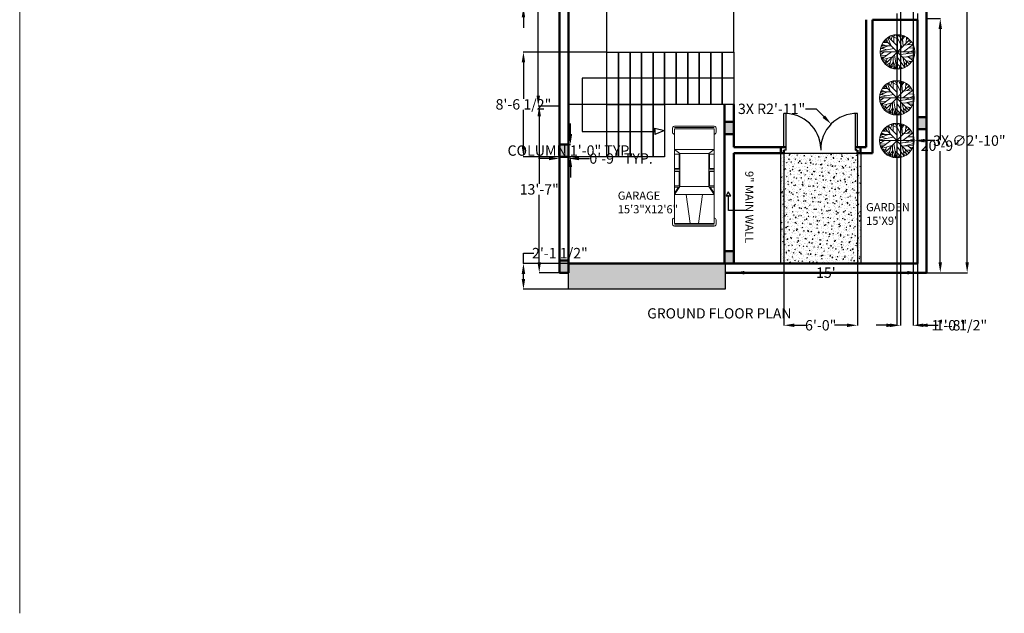
# Model space of a CAD drawing. Units: inches. Extents: x 22 to 1000, y 8 to 1043.
# Tile 1 of 3: x 22 to 987, y 8 to 590. Entities that reach past the tile are written whole.
import ezdxf

# ---------------------------------------------------------------- set-up
doc = ezdxf.new("R2010")
doc.units = ezdxf.units.IN
doc.header["$MEASUREMENT"] = 0
for name, color, linetype, lineweight in [('A-ANNO-DIMS', 2, 'Continuous', 18), ('A-ANNO-TEXT', 7, 'Continuous', 25), ('A-AREA-IDEN', 7, 'Continuous', 25), ('A-COLS', 7, 'Continuous', 50), ('A-COLS-PATT', 1, 'Continuous', 13), ('A-DOOR', 4, 'Continuous', 25), ('A-FLOR-STRS', 7, 'Continuous', 25), ('A-REFR', 8, 'Continuous', 13), ('A-SITE-VEHC', 8, 'Continuous', 18), ('A-WALL', 7, 'Continuous', 50), ('L-PLNT-TREE', 3, 'Continuous', 18), ('L-PVMT', 8, 'Continuous', 25), ('L-PVMT-PATT', 252, 'Continuous', 13)]:
    doc.layers.add(name, color=color, linetype=linetype, lineweight=lineweight)
doc.styles.get("Standard").update_dxf_attribs({"font": 'arial.ttf'})
doc.dimstyles.get("Standard").update_dxf_attribs({"dimtxt": 10.18, "dimasz": 10.18, "dimexe": 0.18, "dimexo": 0.0625, "dimgap": 0.09, "dimtad": 0, "dimtih": 1, "dimtoh": 1, "dimdec": 0, "dimzin": 0, "dimdsep": 46, "dimlunit": 3, "dimtxsty": 'Standard', "dimcen": 0.09, "dimadec": 0, "dimazin": 0, "dimtfac": 1, "dimtdec": 0, "dimtofl": 0, "dimtmove": 0, "dimatfit": 3, "dimfxl": 1, "dimtolj": 1, "dimtzin": 0, "dimarcsym": 0})

# ---------------------------------------------------------------- blocks, each defined once
blk = doc.blocks.new('*U2')
for p, q in [((5.4, 42.3), (12.1, 42.3)), ((189.7, 42.3), (183, 42.3)), ((0.1, -0.4), (0.1, 38.3)), ((2.8, -0.4), (2.8, 38.3)), ((5.4, 38.3), (16.1, 38.3)), ((5.4, -0.4), (5.4, 38.2)), ((16.1, 38.3), (180.3, 38.3)), ((61.5, -0.4), (61.5, 38.3)), ((61.5, 38.3), (77.5, 27.6)), ((64.2, 38.3), (76.2, 30.3)), ((76.2, 30.3), (76.2, 38.3)), ((77.5, 27.6), (141.6, 27.6)), ((77.5, -0.4), (77.5, 27.6)), ((78.9, 38.3), (78.9, 29)), ((78.9, 29), (106.9, 29)), ((106.9, 29), (106.9, 38.3)), ((109.6, 27.6), (109.6, 38.3)), ((112.3, 38.3), (112.3, 29)), ((112.3, 29), (140.3, 29)), ((140.3, 29), (140.3, 38.3)), ((141.6, 27.6), (149.6, 38.3)), ((141.6, -0.4), (141.6, 27.6)), ((149.6, -0.4), (149.6, 38.3)), ((189.7, 38.3), (179, 38.3)), ((189.7, -0.4), (189.7, 38.2)), ((192.4, -0.4), (192.4, 38.3)), ((195, -0.4), (195, 38.3)), ((5.4, 7.6), (61.5, 15.6)), ((0.1, -0.4), (0.1, -39.2)), ((2.8, -0.4), (2.8, -39.1)), ((5.4, -0.4), (5.4, -39.1)), ((5.4, -8.4), (61.5, -16.4)), ((61.5, -0.4), (61.5, -39.1)), ((77.5, -0.4), (77.5, -28.5)), ((141.6, -0.4), (141.6, -28.5)), ((149.6, -0.4), (149.6, -39.1)), ((189.7, -0.4), (189.7, -39.1)), ((192.4, -0.4), (192.4, -39.1)), ((195, -0.4), (195, -39.2)), ((61.5, -39.1), (77.5, -28.5)), ((64.2, -39.1), (76.2, -31.1)), ((76.2, -31.1), (76.2, -39.1)), ((77.5, -28.5), (141.6, -28.5)), ((78.9, -39.1), (78.9, -29.8)), ((78.9, -29.8), (106.9, -29.8)), ((106.9, -29.8), (106.9, -39.1)), ((109.6, -28.5), (109.6, -39.1)), ((112.3, -29.8), (140.3, -29.8)), ((112.3, -39.1), (112.3, -29.8)), ((140.3, -29.8), (140.3, -39.1)), ((141.6, -28.5), (149.6, -39.1)), ((5.4, -39.1), (16.1, -39.1)), ((5.4, -43.1), (12.1, -43.1)), ((16.1, -39.1), (180.3, -39.1)), ((189.7, -39.1), (179, -39.1)), ((189.7, -43.1), (183, -43.1))]:
    blk.add_line(p, q)
for centre, radius, start, end in [((5.1, 37.3), 5.06, 85.6455, 168.0943), ((11.5, 37.6), 4.72, 8.1301, 81.87), ((183.7, 37.6), 4.72, 98.13, 171.8699), ((190.1, 37.3), 5.06, 11.9057, 94.3545), ((5.1, -38.1), 5.06, 191.9057, 274.3545), ((11.5, -38.5), 4.72, 278.13, 351.8699), ((183.7, -38.5), 4.72, 188.1301, 261.87), ((190.1, -38.1), 5.06, 265.6455, 348.0943)]:
    blk.add_arc(centre, radius, start, end)
blk = doc.blocks.new('Tree - deciduous plan')
for p, q in [((-45.8134, 38.2383), (-40.5318, 33.0471)), ((-43.8768, 36.4326), (-44.405, 40.2696)), ((42, 42), (-42, -42)), ((42, -42), (-42, 42)), ((-40.1797, 44.558), (-36.4825, 43.2038)), ((-37.0107, 47.0408), (-35.25, 35.5298)), ((-32.6092, 50.4264), (-23.2782, 23.5674)), ((-31.2008, 51.1035), (-0.2149, 20.1818)), ((-26.4472, 46.5894), (-26.2712, 53.8116)), ((-22.0458, 42.0753), (-16.5881, 57.6486)), ((-21.1656, 55.8436), (-0.0388, 45.0094)), ((-12.5388, 54.9406), (-7.9613, 59.4546)), ((-12.3627, 32.1443), (-12.5388, 58.7776)), ((-5.3205, 59.6806), (16.5105, 16.7963)), ((2.426, 54.9406), (-1.4472, 59.9056)), ((0, 59.9996), (0, -60)), ((0.4894, 48.6208), (3.6584, 59.6806)), ((18.2711, 35.5298), (5.419, 59.6806)), ((9.8203, 51.5549), (12.8133, 58.5516)), ((19.6795, 19.5047), (16.3344, 57.6486)), ((17.0387, 51.1035), (23.2006, 55.1666)), ((17.7429, 43.6552), (25.4894, 54.2636)), ((31.6513, 50.8778), (30.2429, 30.5643)), ((31.1232, 42.5267), (35.8767, 48.1693)), ((36.2288, 25.1474), (48.9049, 35.0784)), ((37.1091, 37.1098), (46.6161, 37.5612)), ((-59.7219, 2.8025), (-12.0106, 12.0565)), ((-32.2571, 20.6333), (-59.1937, 9.348)), ((-58.6656, 12.7336), (-35.9543, 7.5424)), ((-57.081, 17.9248), (-47.0458, 14.7649)), ((-56.0247, 20.859), (-20.8134, 20.859)), ((-54.7923, 24.4702), (-47.75, 21.0847)), ((-54.6162, -24.7335), (-20.2853, 0.0941)), ((-53.2078, 27.4044), (-40.1797, 20.859)), ((-49.8627, 32.8214), (-32.7853, 32.8214)), ((54.3626, 25.3731), (20.9119, 0.3198)), ((23.3767, 23.3417), (53.3063, 27.4044)), ((29.3626, -6.6771), (59.4682, 7.091)), ((38.5175, 13.4107), (58.2359, 13.6364)), ((-60, 0), (60, 0)), ((-59.7219, -4.8714), (-54.2641, -6.6771)), ((-45.2853, -0.1316), (-59.0177, -10.0627)), ((-58.4895, -12.3197), (-36.4825, -11.6426)), ((-57.081, -18.4138), (-45.2853, -17.9624)), ((-52.6797, -18.188), (-55.4966, -22.0251)), ((-53.2078, -27.442), (-16.7641, -16.6081)), ((-38.9472, -29.0219), (-51.4472, -30.6018)), ((-47.2219, -19.3166), (-50.2148, -26.3135)), ((-46.5177, -30.1504), (-49.5106, -33.536)), ((-32.4331, -32.4075), (-48.1021, -35.5674)), ((-35.9543, -22.4765), (-44.0529, -40.5329)), ((-19.9331, -20.2194), (-28.5599, -52.721)), ((-14.8275, -15.0282), (-14.6515, -57.6865)), ((-14.6515, -32.1818), (-3.912, -59.4922)), ((-10.074, -10.0627), (-2.5036, -59.7178)), ((-0.0388, -19.0909), (25.8415, -53.8495)), ((9.2922, -9.1598), (59.6443, -2.8401)), ((18.6232, -18.6394), (26.7218, -53.3981)), ((18.7992, -18.6394), (57.3556, -17.2853)), ((26.3697, -18.4138), (58.9401, -9.8369)), ((30.419, -30.1504), (32.3556, -50.0125)), ((31.4753, -31.279), (49.6091, -33.3103)), ((38.1654, -18.188), (52.426, -29.0219)), ((41.5105, -32.6332), (46.088, -38.0501)), ((45.9119, -24.0564), (55.595, -22.2508)), ((-43.7008, -34.6645), (-46.6937, -37.373)), ((-24.6867, -37.8244), (-38.7712, -45.7241)), ((-26.2712, -43.9185), (-34.7219, -48.6583)), ((-14.6515, -36.2445), (-27.6797, -52.9467)), ((-14.6515, -47.3041), (-25.0388, -54.3009)), ((-21.5177, -45.4984), (-19.9331, -56.1065)), ((-8.4895, -47.5298), (-11.4825, -58.5893)), ((-6.3768, -52.721), (-9.3698, -58.815)), ((-6.2008, -36.2445), (17.919, -57.0094)), ((8.4119, -53.1724), (3.8344, -59.4922)), ((5.9471, -46.6269), (10.5246, -58.5893)), ((22.8485, -36.4702), (35.3485, -48.4326)), ((24.7852, -44.8213), (23.0246, -54.978))]:
    blk.add_line(p, q)
blk.add_circle((0, 0), 60)
blk = doc.blocks.new('*D11')
at = {"layer": 'A-ANNO-DIMS', "color": 0, "lineweight": -2, "transparency": 16777216}
for p, q in [((550.93, 772.66), (530.12, 772.66)), ((530.3, 762.48), (530.3, 644.03)), ((530.3, 515.19), (530.3, 633.63)), ((550.93, 505.01), (530.12, 505.01))]:
    blk.add_line(p, q, dxfattribs=at)
at = {"layer": 'A-ANNO-DIMS', "color": 0, "transparency": 16777216}
for points in [[(528.6, 762.48), (532, 762.48), (530.3, 772.66)], [(528.6, 515.19), (532, 515.19), (530.3, 505.01)]]:
    blk.add_solid(points, dxfattribs=at)
at = {"layer": 'Defpoints', "color": 0, "transparency": 16777216}
for p in [(550.99, 772.66), (530.3, 505.01), (550.99, 505.01)]:
    blk.add_point(p, dxfattribs=at)
at = {"layer": 'A-ANNO-DIMS', "color": 0, "transparency": 16777216, "insert": (530.3, 638.83), "char_height": 10.18, "attachment_point": 5}
blk.add_mtext('\\A1;22\'-4"', dxfattribs=at)
blk = doc.blocks.new('*D12')
at = {"layer": 'A-ANNO-DIMS', "color": 0, "lineweight": -2, "transparency": 16777216}
for p, q in [((550.93, 505.01), (531.04, 505.01)), ((531.22, 494.83), (531.22, 428.62)), ((531.22, 351.84), (531.22, 418.04)), ((550.93, 341.66), (531.04, 341.66))]:
    blk.add_line(p, q, dxfattribs=at)
at = {"layer": 'A-ANNO-DIMS', "color": 0, "transparency": 16777216}
for points in [[(529.52, 494.83), (532.92, 494.83), (531.22, 505.01)], [(529.52, 351.84), (532.92, 351.84), (531.22, 341.66)]]:
    blk.add_solid(points, dxfattribs=at)
at = {"layer": 'Defpoints', "color": 0, "transparency": 16777216}
for p in [(550.99, 505.01), (531.22, 341.66), (550.99, 341.66)]:
    blk.add_point(p, dxfattribs=at)
at = {"layer": 'A-ANNO-DIMS', "color": 0, "transparency": 16777216, "insert": (531.22, 423.33), "char_height": 10.18, "attachment_point": 5}
blk.add_mtext('\\A1;13\'-7"', dxfattribs=at)
blk = doc.blocks.new('*D13')
at = {"layer": 'A-ANNO-DIMS', "color": 0, "lineweight": -2, "transparency": 16777216}
for p, q in [((722.02, 341.72), (722.02, 341.84)), ((732.2, 341.66), (804.01, 341.66)), ((892.32, 341.66), (820.51, 341.66)), ((902.5, 341.72), (902.5, 341.84))]:
    blk.add_line(p, q, dxfattribs=at)
at = {"layer": 'A-ANNO-DIMS', "color": 0, "transparency": 16777216}
for points in [[(732.2, 343.35), (732.2, 339.96), (722.02, 341.66)], [(892.32, 343.35), (892.32, 339.96), (902.5, 341.66)]]:
    blk.add_solid(points, dxfattribs=at)
at = {"layer": 'Defpoints', "color": 0, "transparency": 16777216}
for p in [(722.02, 341.66), (902.5, 341.66), (902.5, 341.66)]:
    blk.add_point(p, dxfattribs=at)
at = {"layer": 'A-ANNO-DIMS', "color": 0, "transparency": 16777216, "insert": (812.26, 341.66), "char_height": 10.18, "attachment_point": 5}
blk.add_mtext("\\A1;15'", dxfattribs=at)
blk = doc.blocks.new('*D14')
at = {"layer": 'A-ANNO-DIMS', "color": 0, "lineweight": -2, "transparency": 16777216}
for p, q in [((911.05, 590.68), (924.64, 590.68)), ((924.46, 580.5), (924.46, 471.45)), ((924.46, 351.84), (924.46, 460.88)), ((911.05, 341.66), (924.64, 341.66))]:
    blk.add_line(p, q, dxfattribs=at)
at = {"layer": 'A-ANNO-DIMS', "color": 0, "transparency": 16777216}
for points in [[(922.77, 580.5), (926.16, 580.5), (924.46, 590.68)], [(922.77, 351.84), (926.16, 351.84), (924.46, 341.66)]]:
    blk.add_solid(points, dxfattribs=at)
at = {"layer": 'Defpoints', "color": 0, "transparency": 16777216}
for p in [(910.99, 590.68), (924.46, 590.68), (910.99, 341.66)]:
    blk.add_point(p, dxfattribs=at)
at = {"layer": 'A-ANNO-DIMS', "color": 0, "transparency": 16777216, "insert": (924.46, 466.17), "char_height": 10.18, "attachment_point": 5}
blk.add_mtext('\\A1;20\'-9"', dxfattribs=at)
blk = doc.blocks.new('*D23')
at = {"layer": 'A-ANNO-DIMS', "color": 0, "lineweight": -2, "transparency": 16777216}
for p, q in [((911.05, 941.29), (951, 941.29)), ((950.82, 931.11), (950.82, 646.76)), ((950.82, 351.84), (950.82, 636.18)), ((911.12, 341.66), (951, 341.66))]:
    blk.add_line(p, q, dxfattribs=at)
at = {"layer": 'A-ANNO-DIMS', "color": 0, "transparency": 16777216}
for points in [[(949.12, 931.11), (952.52, 931.11), (950.82, 941.29)], [(949.12, 351.84), (952.52, 351.84), (950.82, 341.66)]]:
    blk.add_solid(points, dxfattribs=at)
at = {"layer": 'Defpoints', "color": 0, "transparency": 16777216}
for p in [(910.99, 941.29), (911.05, 341.66), (950.82, 341.66)]:
    blk.add_point(p, dxfattribs=at)
at = {"layer": 'A-ANNO-DIMS', "color": 0, "transparency": 16777216, "insert": (950.82, 641.47), "char_height": 10.18, "attachment_point": 5}
blk.add_mtext("\\A1;50'", dxfattribs=at)
blk = doc.blocks.new('COLUMN-9X12IN')
for p, q in [((0, 12), (9, 12)), ((0, 0), (0, 12)), ((9, 12), (9, 0)), ((9, 0), (0, 0))]:
    blk.add_line(p, q)
blk = doc.blocks.new('*D33')
at = {"layer": 'A-ANNO-DIMS', "color": 0, "lineweight": -2, "transparency": 16777216}
for p, q in [((561.79, 477.56), (561.79, 487.74)), ((560.05, 467.38), (561.97, 467.38)), ((560.05, 455.38), (561.97, 455.38)), ((561.79, 445.2), (561.79, 435.02))]:
    blk.add_line(p, q, dxfattribs=at)
at = {"layer": 'A-ANNO-DIMS', "color": 0, "transparency": 16777216}
for points in [[(560.09, 477.56), (563.49, 477.56), (561.79, 467.38)], [(560.09, 445.2), (563.49, 445.2), (561.79, 455.38)]]:
    blk.add_solid(points, dxfattribs=at)
at = {"layer": 'Defpoints', "color": 0, "transparency": 16777216}
for p in [(559.99, 467.38), (561.79, 467.38), (559.99, 455.38)]:
    blk.add_point(p, dxfattribs=at)
at = {"layer": 'A-ANNO-DIMS', "color": 0, "transparency": 16777216, "insert": (561.79, 461.38), "char_height": 10.18, "attachment_point": 5}
blk.add_mtext('\\A1;COLUMN 1\'-0" TYP.', dxfattribs=at)
blk = doc.blocks.new('*D34')
at = {"layer": 'A-ANNO-DIMS', "color": 0, "lineweight": -2, "transparency": 16777216}
for p, q in [((550.99, 455.31), (550.99, 453.4)), ((559.99, 455.31), (559.99, 453.4)), ((540.81, 453.58), (530.63, 453.58)), ((570.17, 453.58), (580.35, 453.58))]:
    blk.add_line(p, q, dxfattribs=at)
at = {"layer": 'A-ANNO-DIMS', "color": 0, "transparency": 16777216}
for points in [[(540.81, 455.27), (540.81, 451.88), (550.99, 453.58)], [(570.17, 455.27), (570.17, 451.88), (559.99, 453.58)]]:
    blk.add_solid(points, dxfattribs=at)
at = {"layer": 'Defpoints', "color": 0, "transparency": 16777216}
for p in [(550.99, 455.38), (559.99, 455.38), (559.99, 453.58)]:
    blk.add_point(p, dxfattribs=at)
at = {"layer": 'A-ANNO-DIMS', "color": 0, "transparency": 16777216, "insert": (611.47, 453.58), "char_height": 10.18, "attachment_point": 5}
blk.add_mtext('\\A1;0\'-9" TYP.', dxfattribs=at)
blk = doc.blocks.new('*D43')
at = {"layer": 'A-ANNO-DIMS', "color": 0, "lineweight": -2, "transparency": 16777216}
for p, q in [((597.67, 558), (597.67, 1028.09)), ((607.85, 1027.91), (630.87, 1027.91)), ((711.81, 1027.91), (688.79, 1027.91)), ((721.99, 558), (721.99, 1028.09))]:
    blk.add_line(p, q, dxfattribs=at)
at = {"layer": 'A-ANNO-DIMS', "color": 0, "transparency": 16777216}
for points in [[(607.85, 1029.6), (607.85, 1026.21), (597.67, 1027.91)], [(711.81, 1029.6), (711.81, 1026.21), (721.99, 1027.91)]]:
    blk.add_solid(points, dxfattribs=at)
at = {"layer": 'Defpoints', "color": 0, "transparency": 16777216}
for p in [(721.99, 1027.91), (597.67, 557.94), (721.99, 557.94)]:
    blk.add_point(p, dxfattribs=at)
at = {"layer": 'A-ANNO-DIMS', "color": 0, "transparency": 16777216, "insert": (659.83, 1027.91), "char_height": 10.18, "attachment_point": 5}
blk.add_mtext('\\A1;10\'-4 1/2"', dxfattribs=at)
blk = doc.blocks.new('*D44')
at = {"layer": 'A-ANNO-DIMS', "color": 0, "lineweight": -2, "transparency": 16777216}
for p, q in [((597.61, 557.94), (515.56, 557.94)), ((515.74, 547.76), (515.74, 512.01)), ((515.74, 465.56), (515.74, 501.3)), ((597.61, 455.38), (515.56, 455.38))]:
    blk.add_line(p, q, dxfattribs=at)
at = {"layer": 'A-ANNO-DIMS', "color": 0, "transparency": 16777216}
for points in [[(514.04, 547.76), (517.44, 547.76), (515.74, 557.94)], [(514.04, 465.56), (517.44, 465.56), (515.74, 455.38)]]:
    blk.add_solid(points, dxfattribs=at)
at = {"layer": 'Defpoints', "color": 0, "transparency": 16777216}
for p in [(515.74, 557.94), (597.67, 557.94), (597.67, 455.38)]:
    blk.add_point(p, dxfattribs=at)
at = {"layer": 'A-ANNO-DIMS', "color": 0, "transparency": 16777216, "insert": (515.74, 506.66), "char_height": 10.18, "attachment_point": 5}
blk.add_mtext('\\A1;8\'-6 1/2"', dxfattribs=at)
blk = doc.blocks.new('*D45')
at = {"layer": 'A-ANNO-DIMS', "color": 0, "lineweight": -2, "transparency": 16777216}
for p, q in [((771.22, 458.59), (771.22, 289.9)), ((843.22, 458.59), (843.22, 289.9)), ((781.4, 290.08), (793.57, 290.08)), ((833.04, 290.08), (820.87, 290.08))]:
    blk.add_line(p, q, dxfattribs=at)
at = {"layer": 'A-ANNO-DIMS', "color": 0, "transparency": 16777216}
for points in [[(781.4, 291.77), (781.4, 288.38), (771.22, 290.08)], [(833.04, 291.77), (833.04, 288.38), (843.22, 290.08)]]:
    blk.add_solid(points, dxfattribs=at)
at = {"layer": 'Defpoints', "color": 0, "transparency": 16777216}
for p in [(771.22, 458.66), (843.22, 458.66), (843.22, 290.08)]:
    blk.add_point(p, dxfattribs=at)
at = {"layer": 'A-ANNO-DIMS', "color": 0, "transparency": 16777216, "insert": (807.22, 290.08), "char_height": 10.18, "attachment_point": 5}
blk.add_mtext('\\A1;6\'-0"', dxfattribs=at)
blk = doc.blocks.new('*D48')
at = {"layer": 'A-ANNO-DIMS', "color": 0, "lineweight": -2, "transparency": 16777216}
for p, q in [((881.83, 595.59), (881.83, 289.9)), ((901.99, 595.59), (901.99, 289.9)), ((871.65, 290.08), (861.47, 290.08)), ((912.17, 290.08), (922.35, 290.08))]:
    blk.add_line(p, q, dxfattribs=at)
at = {"layer": 'A-ANNO-DIMS', "color": 0, "transparency": 16777216}
for points in [[(871.65, 291.77), (871.65, 288.38), (881.83, 290.08)], [(912.17, 291.77), (912.17, 288.38), (901.99, 290.08)]]:
    blk.add_solid(points, dxfattribs=at)
at = {"layer": 'Defpoints', "color": 0, "transparency": 16777216}
for p in [(881.83, 595.66), (901.99, 595.66), (901.99, 290.08)]:
    blk.add_point(p, dxfattribs=at)
at = {"layer": 'A-ANNO-DIMS', "color": 0, "transparency": 16777216, "insert": (935.49, 290.08), "char_height": 10.18, "attachment_point": 5}
blk.add_mtext('\\A1;1\'-8"', dxfattribs=at)
blk = doc.blocks.new('*D50')
at = {"layer": 'A-ANNO-DIMS', "color": 0, "lineweight": -2, "transparency": 16777216}
for p, q in [((885.49, 605.07), (885.49, 289.9)), ((897.78, 605.07), (897.78, 289.9)), ((875.31, 290.08), (865.13, 290.08)), ((907.96, 290.08), (918.14, 290.08))]:
    blk.add_line(p, q, dxfattribs=at)
at = {"layer": 'A-ANNO-DIMS', "color": 0, "transparency": 16777216}
for points in [[(875.31, 291.77), (875.31, 288.38), (885.49, 290.08)], [(907.96, 291.77), (907.96, 288.38), (897.78, 290.08)]]:
    blk.add_solid(points, dxfattribs=at)
at = {"layer": 'Defpoints', "color": 0, "transparency": 16777216}
for p in [(885.49, 605.13), (897.78, 605.13), (897.78, 290.08)]:
    blk.add_point(p, dxfattribs=at)
at = {"layer": 'A-ANNO-DIMS', "color": 0, "transparency": 16777216, "insert": (943.14, 290.08), "char_height": 10.18, "attachment_point": 5}
blk.add_mtext('\\A1;1\'-0 1/2"', dxfattribs=at)
blk = doc.blocks.new('*D51')
at = {"layer": 'A-ANNO-DIMS', "color": 0, "lineweight": -2, "transparency": 16777216}
for p, q in [((515.74, 625.87), (515.74, 636.05)), ((888.43, 615.69), (515.56, 615.69)), ((888.43, 602.13), (515.56, 602.13)), ((515.74, 591.95), (515.74, 581.77))]:
    blk.add_line(p, q, dxfattribs=at)
at = {"layer": 'A-ANNO-DIMS', "color": 0, "transparency": 16777216}
for points in [[(514.04, 625.87), (517.44, 625.87), (515.74, 615.69)], [(514.04, 591.95), (517.44, 591.95), (515.74, 602.13)]]:
    blk.add_solid(points, dxfattribs=at)
at = {"layer": 'Defpoints', "color": 0, "transparency": 16777216}
for p in [(515.74, 615.69), (888.49, 615.69), (888.49, 602.13)]:
    blk.add_point(p, dxfattribs=at)
at = {"layer": 'A-ANNO-DIMS', "color": 0, "transparency": 16777216, "insert": (515.74, 608.91), "char_height": 10.18, "attachment_point": 5}
blk.add_mtext('\\A1;1\'-1 1/2"', dxfattribs=at)
blk = doc.blocks.new('*D57')
at = {"layer": 'A-ANNO-DIMS', "color": 0, "lineweight": -2, "transparency": 16777216}
for p, q in [((515.74, 350.66), (515.74, 360.84)), ((515.74, 360.84), (525.92, 360.84)), ((559.93, 350.66), (515.56, 350.66)), ((515.74, 335.51), (515.74, 340.48)), ((559.93, 325.33), (515.56, 325.33))]:
    blk.add_line(p, q, dxfattribs=at)
at = {"layer": 'A-ANNO-DIMS', "color": 0, "transparency": 16777216}
for points in [[(514.04, 340.48), (517.44, 340.48), (515.74, 350.66)], [(514.04, 335.51), (517.44, 335.51), (515.74, 325.33)]]:
    blk.add_solid(points, dxfattribs=at)
at = {"layer": 'Defpoints', "color": 0, "transparency": 16777216}
for p in [(515.74, 350.66), (559.99, 350.66), (559.99, 325.33)]:
    blk.add_point(p, dxfattribs=at)
at = {"layer": 'A-ANNO-DIMS', "color": 0, "transparency": 16777216, "insert": (551.49, 360.84), "char_height": 10.18, "attachment_point": 5}
blk.add_mtext('\\A1;2\'-1 1/2"', dxfattribs=at)
blk = doc.blocks.new('*D58')
at = {"layer": 'A-ANNO-DIMS', "color": 0, "lineweight": -2, "transparency": 16777216}
for p, q in [((792.43, 502.27), (802.61, 502.27)), ((802.61, 502.27), (810.26, 494.61)), ((842.13, 462.66), (842.31, 462.66)), ((842.22, 462.57), (842.22, 462.75))]:
    blk.add_line(p, q, dxfattribs=at)
at = {"layer": 'A-ANNO-DIMS', "color": 0, "transparency": 16777216}
blk.add_solid([(811.46, 495.81), (809.06, 493.41), (817.46, 487.42)], dxfattribs=at)
at = {"layer": 'Defpoints', "color": 0, "transparency": 16777216}
for p in [(817.46, 487.42), (842.22, 462.66)]:
    blk.add_point(p, dxfattribs=at)
at = {"layer": 'A-ANNO-DIMS', "color": 0, "transparency": 16777216, "insert": (759.05, 502.27), "char_height": 10.18, "attachment_point": 5}
blk.add_mtext('\\A1;3X R2\'-11"', dxfattribs=at)
blk = doc.blocks.new('*D62')
at = {"layer": 'A-ANNO-DIMS', "color": 0, "lineweight": -2, "transparency": 16777216}
for p, q in [((881.77, 471.1), (881.95, 471.1)), ((881.86, 471.01), (881.86, 471.19)), ((919.21, 471.1), (909.03, 471.1))]:
    blk.add_line(p, q, dxfattribs=at)
at = {"layer": 'A-ANNO-DIMS', "color": 0, "transparency": 16777216}
blk.add_solid([(909.03, 472.8), (909.03, 469.4), (898.85, 471.1)], dxfattribs=at)
at = {"layer": 'Defpoints', "color": 0, "transparency": 16777216}
for p in [(864.87, 471.1), (898.85, 471.1)]:
    blk.add_point(p, dxfattribs=at)
at = {"layer": 'A-ANNO-DIMS', "color": 0, "transparency": 16777216, "insert": (952.99, 471.1), "char_height": 10.18, "attachment_point": 5}
blk.add_mtext('\\A1;3X ∅2\'-10"', dxfattribs=at)

msp = doc.modelspace()

# ---------------------------------------------------------------- hatches: boundary and pattern name
at = {"layer": 'A-COLS-PATT'}
h = msp.add_hatch(color=256, dxfattribs=at)
h.dxf.hatch_style = 1
h.paths.add_polyline_path([(559.99, 941.66), (550.99, 941.66), (550.99, 929.67), (559.99, 929.67)])
h.paths.add_polyline_path([(910.99, 941.29), (901.99, 941.29), (901.99, 929.29), (910.99, 929.29)])
h.paths.add_polyline_path([(910.99, 783.96), (901.99, 783.96), (901.99, 771.96), (910.99, 771.96)])
h.paths.add_polyline_path([(910.99, 693.33), (901.99, 693.33), (901.99, 681.33), (910.99, 681.33)])
h.paths.add_polyline_path([(910.99, 494.22), (901.99, 494.22), (901.99, 482.22), (910.99, 482.22)])
h.paths.add_polyline_path([(721.99, 362.66), (712.99, 362.66), (712.99, 350.66), (721.99, 350.66)])
h.paths.add_polyline_path([(721.99, 489.46), (712.99, 489.46), (712.99, 477.46), (721.99, 477.46)])
h.paths.add_polyline_path([(559.99, 353.66), (550.99, 353.66), (550.99, 341.66), (559.99, 341.66)])
h.paths.add_polyline_path([(559.99, 467.38), (550.99, 467.38), (550.99, 455.38), (559.99, 455.38)])
h.paths.add_polyline_path([(559.99, 784.66), (550.99, 784.66), (550.99, 772.66), (559.99, 772.66)])
h.paths.add_polyline_path([(715.99, 781.66), (712.99, 781.66), (712.99, 784.66), (706.99, 784.66), (706.99, 772.66), (715.99, 772.66)])
h.paths.add_polyline_path([(822.98, 688.66), (813.98, 688.66), (813.98, 676.66), (819.92, 676.66), (819.92, 682.66), (822.98, 682.66)])
at = {"layer": 'L-PVMT-PATT'}
h = msp.add_hatch(dxfattribs=at)
h.set_pattern_fill('AR-CONC', color=256)
h.set_pattern_definition([(50, (0, 0), (7.172602, -0.62752), [0.75, -8.25]), (355, (0, 0), (-1.387513, 7.52192), [0.6, -6.6]), (100.45144, (0.598, -0.052), (5.78509, 6.8944), [0.6374, -7.01142]), (46.1842, (0, 2), (10.67241, -1.65519), [1.125, -12.375]), (96.6356, (0.889, 1.862), (9.34662, 9.74119), [0.9561, -10.51714]), (351.1842, (0, 2), (9.34662, 9.74119), [0.9, -9.9]), (21, (1, 1.5), (5.96907, -4.02619), [0.75, -8.25]), (326, (1, 1.5), (2.433153, 7.2515), [0.6, -6.6]), (71.45144, (1.4974, 1.1645), (8.402224, 3.22531), [0.6374, -7.01142]), (37.5, (0, 0), (0.1215986, 3.3289385), [0, -6.52, 0, -6.7, 0, -6.625]), (7.5, (0, 0), (2.630695, 3.944117), [0, -3.82, 0, -6.37, 0, -2.525]), (327.5, (-2.23, 0), (5.338224, -0.225549), [0, -2.5, 0, -7.8, 0, -10.35]), (317.5, (-3.23, 0), (5.831862, 1.00105), [0, -3.25, 0, -5.18, 0, -7.35])])
h.paths.add_polyline_path([(846.47, 458.66), (768.22, 458.66), (768.22, 350.66), (846.47, 350.66)])
h = msp.add_hatch(color=256, dxfattribs=at)
h.dxf.hatch_style = 1
h.paths.add_polyline_path([(713.65, 350.66), (559.99, 350.66), (559.99, 325.33), (713.65, 325.33)])

# ---------------------------------------------------------------- linework, layer by layer
at = {"layer": 'A-ANNO-TEXT'}
for p, q in [((716.6, 421.05), (714.6, 417.05)), ((716.89, 417.05), (714.6, 417.05)), ((714.6, 417.05), (719.03, 417.05)), ((719.03, 417.05), (716.6, 421.05)), ((716.89, 402.52), (716.89, 417.05)), ((733.07, 402.52), (716.89, 402.52))]:
    msp.add_line(p, q, dxfattribs=at)
at = {"layer": 'A-DOOR'}
for p, q in [((771.22, 464.66), (771.22, 497.66)), ((773.22, 461.66), (773.22, 497.66)), ((841.22, 461.66), (841.22, 497.66)), ((843.22, 464.66), (843.22, 497.66)), ((807.26, 464.66), (807.18, 464.66)), ((807.22, 464.66), (807.22, 461.66)), ((773.22, 461.66), (771.22, 461.66)), ((841.22, 461.66), (843.22, 461.66))]:
    msp.add_line(p, q, dxfattribs=at)
for centre, start, end in [((772.22, 462.66), 1.63658, 91.63658), ((842.22, 462.66), 88.36342, 181.63658)]:
    msp.add_arc(centre, 35.01, start, end, dxfattribs=at)
at = {"layer": 'A-FLOR-STRS'}
for p, q in [((721.99, 532.3), (573.24, 532.3)), ((573.24, 532.3), (573.24, 480.19)), ((721.99, 506.66), (559.99, 506.66)), ((644.59, 480.19), (644.59, 483.37)), ((644.59, 483.37), (644.59, 476.98)), ((644.59, 483.37), (654.18, 481.02)), ((573.24, 480.19), (644.59, 480.19)), ((654.18, 481.02), (644.59, 476.98)), ((597.67, 455.38), (559.99, 455.38))]:
    msp.add_line(p, q, dxfattribs=at)
for points in [[(608.97, 506.66), (597.67, 506.66), (597.67, 557.94), (608.97, 557.94)], [(620.27, 506.66), (608.97, 506.66), (608.97, 557.94), (620.27, 557.94)], [(631.57, 506.66), (620.27, 506.66), (620.27, 557.94), (631.57, 557.94)], [(642.88, 506.66), (631.57, 506.66), (631.57, 557.94), (642.88, 557.94)], [(654.18, 506.66), (642.88, 506.66), (642.88, 557.94), (654.18, 557.94)], [(665.48, 506.66), (654.18, 506.66), (654.18, 557.94), (665.48, 557.94)], [(676.78, 506.66), (665.48, 506.66), (665.48, 557.94), (676.78, 557.94)], [(688.08, 506.66), (676.78, 506.66), (676.78, 557.94), (688.08, 557.94)], [(699.39, 506.66), (688.08, 506.66), (688.08, 557.94), (699.39, 557.94)], [(710.69, 506.66), (699.39, 506.66), (699.39, 557.94), (710.69, 557.94)], [(721.99, 506.66), (710.69, 506.66), (710.69, 557.94), (721.99, 557.94)], [(608.97, 455.38), (597.67, 455.38), (597.67, 506.66), (608.97, 506.66)], [(620.27, 455.38), (608.97, 455.38), (608.97, 506.66), (620.27, 506.66)], [(631.57, 455.38), (620.27, 455.38), (620.27, 506.66), (631.57, 506.66)], [(642.88, 455.38), (631.57, 455.38), (631.57, 506.66), (642.88, 506.66)], [(654.18, 455.38), (642.88, 455.38), (642.88, 506.66), (654.18, 506.66)]]:
    msp.add_lwpolyline(points, close=True, dxfattribs=at)
at = {"layer": 'A-REFR'}
msp.add_line((21.79, 7.73), (21.79, 607.73), dxfattribs=at)
at = {"layer": 'A-WALL'}
for p, q in [((550.99, 341.66), (550.99, 941.66)), ((910.99, 941.66), (910.99, 341.66)), ((559.99, 506.66), (559.99, 772.66)), ((851.96, 589.66), (851.96, 464.66)), ((857.96, 589.66), (857.96, 458.66)), ((857.96, 589.66), (901.99, 589.66)), ((901.99, 589.66), (901.99, 350.66)), ((559.99, 350.66), (559.99, 506.66)), ((712.99, 506.66), (712.99, 350.66)), ((721.99, 506.66), (721.99, 464.66)), ((773.22, 464.66), (721.99, 464.66)), ((768.22, 464.66), (768.22, 458.66)), ((851.96, 464.66), (841.22, 464.66)), ((846.22, 464.66), (846.22, 458.66)), ((721.99, 458.66), (721.99, 350.66)), ((771.22, 458.66), (721.99, 458.66)), ((771.22, 461.66), (771.22, 458.66)), ((843.22, 461.66), (843.22, 458.66)), ((857.96, 458.66), (843.22, 458.66)), ((901.99, 458.66), (901.99, 350.66)), ((712.99, 350.66), (559.99, 350.66)), ((901.99, 350.66), (721.99, 350.66)), ((559.99, 341.66), (550.99, 341.66)), ((910.99, 341.66), (713.65, 341.66))]:
    msp.add_line(p, q, dxfattribs=at)
at = {"layer": 'L-PVMT'}
for points in [[(768.22, 458.66), (846.47, 458.66), (846.47, 350.66), (768.22, 350.66)], [(559.99, 350.66), (713.65, 350.66), (713.65, 325.33), (559.99, 325.33)]]:
    msp.add_lwpolyline(points, close=True, dxfattribs=at)

# ---------------------------------------------------------------- block references
at = {"layer": 'A-COLS'}
for p in [(901.99, 482.22), (712.99, 477.46), (550.99, 455.38), (712.99, 350.66), (550.99, 341.66)]:
    msp.add_blockref('COLUMN-9X12IN', p, dxfattribs=at)
at = {"layer": 'A-SITE-VEHC', "xscale": 0.5026625088045467, "yscale": 0.5026625088045467, "zscale": 0.5026625088045467, "rotation": 90}
msp.add_blockref('*U2', (683.06, 387.27), dxfattribs=at)
at = {"layer": 'L-PLNT-TREE', "xscale": 0.2831773886642335, "yscale": 0.2831773886642335, "zscale": 0.2831773886642335}
for p in [(882.43, 558.06), (881.86, 512.98), (881.86, 471.1)]:
    msp.add_blockref('Tree - deciduous plan', p, dxfattribs=at)

# ---------------------------------------------------------------- texts
at = {"layer": 'A-ANNO-TEXT', "insert": (741.24, 441.35), "char_height": 8, "attachment_point": 1, "rotation": 270}
msp.add_mtext_dynamic_manual_height_columns('9" MAIN WALL', width=74.8979, gutter_width=1, heights=[0], dxfattribs=at)
at = {"layer": 'A-ANNO-TEXT', "insert": (637.12, 306.76), "char_height": 10, "attachment_point": 1}
msp.add_mtext_dynamic_manual_height_columns('GROUND FLOOR PLAN', width=336.5001, gutter_width=1, heights=[0], dxfattribs=at)
at = {"layer": 'A-AREA-IDEN', "char_height": 8, "attachment_point": 1}
for s, insert in [('GARAGE\\P15\'3"X12\'6"', (608.23, 421.16)), ("GARDEN \\P15'X9'", (851.7, 409.88))]:
    msp.add_mtext_dynamic_manual_height_columns(s, width=46.5585, gutter_width=1, heights=[0], dxfattribs=dict(at, insert=insert))

# ---------------------------------------------------------------- dimensions: what is measured, and where the dimension line sits
at = {"layer": 'A-ANNO-DIMS'}
for base, p1, p2, override, picture, middle in [((721.99, 1027.91), (597.67, 557.94), (721.99, 557.94), {"dimdec": 1, "dimlfac": 1, "dimrnd": 0, "dimzin": 1, "dimdsep": 46, "dimlunit": 4, "dimfrac": 2}, '*D43', (659.83, 1027.91)), ((897.78, 290.08), (885.49, 605.13), (897.78, 605.13), {"dimdec": 1, "dimlfac": 1, "dimrnd": 0, "dimzin": 1, "dimdsep": 46, "dimlunit": 4, "dimfrac": 2}, '*D50', (943.14, 290.08)), ((901.99, 290.08), (881.83, 595.66), (901.99, 595.66), {"dimdec": 1, "dimlfac": 1, "dimrnd": 0, "dimzin": 1, "dimdsep": 46, "dimlunit": 4, "dimfrac": 2}, '*D48', (935.49, 290.08)), ((843.22, 290.08), (771.22, 458.66), (843.22, 458.66), {"dimdec": 1, "dimlfac": 1, "dimrnd": 0, "dimzin": 1, "dimdsep": 46, "dimlunit": 4, "dimfrac": 2}, '*D45', (807.22, 290.08)), ((902.5, 341.66), (722.02, 341.66), (902.5, 341.66), {"dimclrd": 0, "dimclre": 0, "dimclrt": 0}, '*D13', (812.26, 341.66))]:
    dim = msp.add_linear_dim(base=base, p1=p1, p2=p2, dimstyle='Standard', override=override, dxfattribs=at)
    dim.commit()
    dim.dimension.update_dxf_attribs({"geometry": picture, "text_midpoint": middle})
for base, p1, p2, override, picture, middle in [((950.82, 341.66), (910.99, 941.29), (911.05, 341.66), {"dimclrd": 0, "dimclre": 0, "dimclrt": 0}, '*D23', (950.82, 641.47)), ((530.3, 505.01), (550.99, 772.66), (550.99, 505.01), {"dimclrd": 0, "dimclre": 0, "dimclrt": 0}, '*D11', (530.3, 638.83)), ((515.74, 615.69), (888.49, 602.13), (888.49, 615.69), {"dimdec": 1, "dimlfac": 1, "dimrnd": 0, "dimzin": 1, "dimdsep": 46, "dimlunit": 4, "dimfrac": 2}, '*D51', (515.74, 608.91)), ((924.46, 590.68), (910.99, 341.66), (910.99, 590.68), {"dimclrd": 0, "dimclre": 0, "dimclrt": 0}, '*D14', (924.46, 466.17)), ((515.74, 557.94), (597.67, 455.38), (597.67, 557.94), {"dimdec": 1, "dimlfac": 1, "dimrnd": 0, "dimzin": 1, "dimdsep": 46, "dimlunit": 4, "dimfrac": 2}, '*D44', (515.74, 506.66)), ((531.22, 341.66), (550.99, 505.01), (550.99, 341.66), {"dimclrd": 0, "dimclre": 0, "dimclrt": 0}, '*D12', (531.22, 423.33)), ((515.74, 350.66), (559.99, 325.33), (559.99, 350.66), {"dimdec": 1, "dimlfac": 1, "dimrnd": 0, "dimzin": 1, "dimdsep": 46, "dimlunit": 4, "dimfrac": 2}, '*D57', (551.49, 360.84))]:
    dim = msp.add_linear_dim(base=base, p1=p1, p2=p2, angle=90, dimstyle='Standard', override=override, dxfattribs=at)
    dim.commit()
    dim.dimension.update_dxf_attribs({"geometry": picture, "text_midpoint": middle})
dim = msp.add_radius_dim(center=(842.22, 462.66), mpoint=(817.46, 487.42), text='3X <>', dimstyle='Standard', override={"dimdec": 1, "dimlfac": 1, "dimrnd": 0, "dimzin": 1, "dimdsep": 46, "dimlunit": 4, "dimfrac": 2}, dxfattribs=at)
dim.commit()
dim.dimension.update_dxf_attribs({"geometry": '*D58', "text_midpoint": (759.05, 502.27), "dimtype": 164})
dim = msp.add_linear_dim(base=(561.79, 467.38), p1=(559.99, 455.38), p2=(559.99, 467.38), angle=90, text='COLUMN <> TYP.', dimstyle='Standard', override={"dimdec": 1, "dimlfac": 1, "dimrnd": 0, "dimzin": 1, "dimdsep": 46, "dimlunit": 4, "dimfrac": 2}, dxfattribs=at)
dim.commit()
dim.dimension.update_dxf_attribs({"geometry": '*D33', "text_midpoint": (561.79, 461.38)})
dim = msp.add_diameter_dim_2p(p1=(864.87, 471.1), p2=(898.85, 471.1), text='3X <>', dimstyle='Standard', override={"dimdec": 1, "dimlfac": 1, "dimrnd": 0, "dimzin": 1, "dimdsep": 46, "dimlunit": 4, "dimfrac": 2}, dxfattribs=at)
dim.commit()
dim.dimension.update_dxf_attribs({"geometry": '*D62', "text_midpoint": (919.21, 471.1)})
dim = msp.add_linear_dim(base=(559.99, 453.58), p1=(550.99, 455.38), p2=(559.99, 455.38), text='<> TYP.', dimstyle='Standard', override={"dimdec": 1, "dimlfac": 1, "dimrnd": 0, "dimzin": 1, "dimdsep": 46, "dimlunit": 4, "dimfrac": 2}, dxfattribs=at)
dim.commit()
dim.dimension.update_dxf_attribs({"geometry": '*D34', "text_midpoint": (611.47, 453.58)})

doc.saveas('drawing.dxf')
